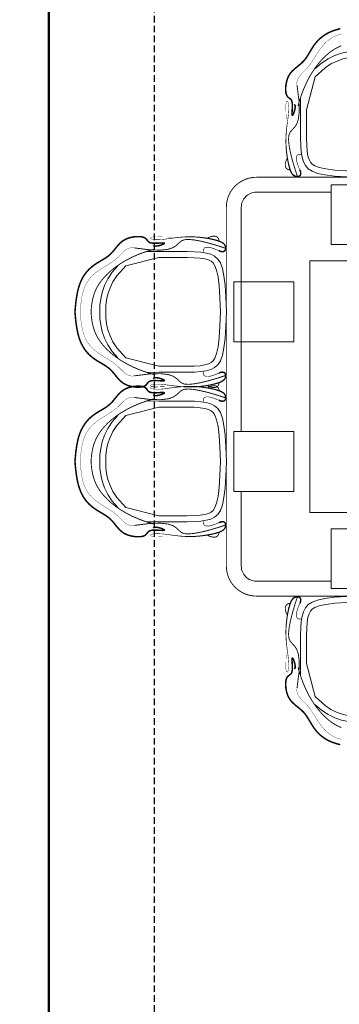
# Model space of a CAD drawing. Units: inches. Extents: x 513 to 1142, y 396 to 927.
# Tile 20 of 31: x 838 to 862, y 691 to 766. Entities that reach past the tile are written whole.
import ezdxf

# ---------------------------------------------------------------- set-up
doc = ezdxf.new("R2010")
doc.units = ezdxf.units.IN
doc.header["$MEASUREMENT"] = 0
doc.linetypes.add('DASHED', pattern=[0.75, 0.5, -0.25])
for name, color, linetype, lineweight in [('A-ANNO-DIMS', 2, 'DASHED', 18), ('A-WALL', 7, 'Continuous', 50), ('furniture', 92, 'Continuous', 18)]:
    doc.layers.add(name, color=color, linetype=linetype, lineweight=lineweight)
doc.styles.get("Standard").update_dxf_attribs({"font": 'arial.ttf'})
doc.dimstyles.get("Standard").update_dxf_attribs({"dimtxt": 4, "dimasz": 0.18, "dimexe": 0.18, "dimexo": 0.0625, "dimgap": 0.09, "dimtad": 0, "dimtih": 1, "dimtoh": 1, "dimdec": 0, "dimrnd": 6, "dimzin": 0, "dimdsep": 46, "dimlunit": 3, "dimtxsty": 'Standard', "dimcen": 0.09, "dimadec": 0, "dimazin": 0, "dimtfac": 1, "dimtdec": 0, "dimtofl": 0, "dimtmove": 0, "dimatfit": 3, "dimfxl": 1, "dimtolj": 1, "dimtzin": 0, "dimarcsym": 0})

# ---------------------------------------------------------------- blocks, each defined once
blk = doc.blocks.new('ОГ55_на6персон_стол1400х900')
for points, const_width in [([(-473.4, 523.4), (-471.2, 521.4), (-470.1, 518.2), (-469.9, 514.2), (-470.4, 509.6), (-471.4, 504.8), (-472.7, 500.1), (-474.2, 495.7), (-475.7, 492), (-477, 489.2), (-478, 487.3), (-478.9, 486.4), (-479.6, 486.4), (-480.1, 487.3), (-480.4, 489.1), (-480.6, 491.8), (-480.5, 495.4), (-480.3, 499.8), (-480, 504.9), (-479.7, 510.3), (-479.6, 516), (-479.6, 521.5), (-479.9, 526.8), (-480.6, 531.5), (-481.8, 535.5), (-483.5, 538.5), (-485.7, 540.8), (-488.2, 542.8), (-490.8, 544.6), (-493.4, 546.7), (-495.9, 549.3), (-498.1, 552.7), (-499.8, 557.2), (-501.1, 563.1), (-501.7, 570.2), (-501.7, 578.1), (-501, 586.6), (-499.6, 595.4), (-497.4, 604.2), (-494.3, 612.7), (-490.4, 620.6), (-485.5, 627.7), (-480, 634.2), (-473.9, 640.1), (-467.5, 645.6), (-460.9, 650.9), (-454.3, 656.2), (-448.1, 661.7), (-442.2, 667.5), (-436.9, 673.7), (-432.1, 680.3), (-427.6, 687.3), (-423.2, 694.5), (-418.9, 701.9), (-414.4, 709.4), (-409.5, 716.9), (-404.2, 724.4), (-398.3, 731.7), (-391.7, 738.8), (-384.3, 745.6), (-376.1, 752), (-366.9, 758), (-356.7, 763.4), (-345.4, 768.3), (-333, 772.5), (-319.5, 776), (-305.4, 778.8), (-291.5, 780.9), (-278.6, 782.6), (-267.2, 783.7), (-258.2, 784.5), (-252.2, 784.9), (-250, 785)], 5), ([(-463.8, 586.5), (-464.6, 595.2), (-463.4, 603), (-460.5, 610.1), (-456.3, 616.6), (-451.1, 622.8), (-445.3, 628.7), (-439.3, 634.6), (-433.4, 640.6), (-427.9, 646.8), (-422.8, 653.3), (-417.9, 659.9), (-413.3, 666.7), (-408.8, 673.7), (-404.4, 680.7), (-400, 687.9), (-395.5, 695), (-390.8, 702.2), (-385.8, 709.3), (-380.5, 716.3), (-374.7, 723.1), (-368.5, 729.6), (-361.7, 735.7), (-354.1, 741.4), (-345.9, 746.6), (-336.7, 751.2), (-326.7, 755.2), (-315.5, 758.7), (-303.3, 761.5), (-289.8, 763.8), (-274.9, 765.6), (-258.6, 766.8), (-250, 767.1)], 1), ([(-26.6, 523.4), (-28.8, 521.4), (-29.9, 518.2), (-30.1, 514.2), (-29.6, 509.6), (-28.6, 504.8), (-27.3, 500.1), (-25.8, 495.7), (-24.3, 492), (-23, 489.2), (-22, 487.3), (-21.1, 486.4), (-20.4, 486.4), (-19.9, 487.3), (-19.6, 489.1), (-19.4, 491.8), (-19.5, 495.4), (-19.7, 499.8), (-20, 504.9), (-20.3, 510.3), (-20.4, 516), (-20.4, 521.5), (-20.1, 526.8), (-19.4, 531.5), (-18.2, 535.5), (-16.5, 538.5), (-14.3, 540.8), (-11.8, 542.8), (-9.2, 544.6), (-6.6, 546.7), (-4.1, 549.3), (-1.9, 552.7), (-0.2, 557.2), (1.1, 563.1), (1.7, 570.2), (1.7, 578.1), (1, 586.6), (-0.4, 595.4), (-2.6, 604.2), (-5.7, 612.7), (-9.6, 620.6), (-14.5, 627.7), (-20, 634.2), (-26.1, 640.1), (-32.5, 645.6), (-39.1, 650.9), (-45.7, 656.2), (-51.9, 661.7), (-57.8, 667.5), (-63.1, 673.7), (-67.9, 680.3), (-72.4, 687.3), (-76.8, 694.5), (-81.1, 701.9), (-85.6, 709.4), (-90.5, 716.9), (-95.8, 724.4), (-101.7, 731.7), (-108.3, 738.8), (-115.7, 745.6), (-123.9, 752), (-133.1, 758), (-143.3, 763.4), (-154.6, 768.3), (-167, 772.5), (-180.5, 776), (-194.6, 778.8), (-208.5, 780.9), (-221.4, 782.6), (-232.8, 783.7), (-241.8, 784.5), (-247.8, 784.9), (-250, 785)], 5), ([(-36.2, 586.5), (-35.4, 595.2), (-36.6, 603), (-39.5, 610.1), (-43.7, 616.6), (-48.9, 622.8), (-54.7, 628.7), (-60.7, 634.6), (-66.6, 640.6), (-72.1, 646.8), (-77.2, 653.3), (-82.1, 659.9), (-86.7, 666.7), (-91.2, 673.7), (-95.6, 680.7), (-100, 687.9), (-104.5, 695), (-109.2, 702.2), (-114.2, 709.3), (-119.5, 716.3), (-125.3, 723.1), (-131.5, 729.6), (-138.3, 735.7), (-145.9, 741.4), (-154.1, 746.6), (-163.3, 751.2), (-173.3, 755.2), (-184.5, 758.7), (-196.7, 761.5), (-210.2, 763.8), (-225.1, 765.6), (-241.4, 766.8), (-250, 767.1)], 1), ([(26.6, 523.4), (28.8, 521.4), (29.9, 518.2), (30.1, 514.2), (29.6, 509.6), (28.6, 504.8), (27.3, 500.1), (25.8, 495.7), (24.3, 492), (23, 489.2), (22, 487.3), (21.1, 486.4), (20.4, 486.4), (19.9, 487.3), (19.6, 489.1), (19.4, 491.8), (19.5, 495.4), (19.7, 499.8), (20, 504.9), (20.3, 510.3), (20.4, 516), (20.4, 521.5), (20.1, 526.8), (19.4, 531.5), (18.2, 535.5), (16.5, 538.5), (14.3, 540.8), (11.8, 542.8), (9.2, 544.6), (6.6, 546.7), (4.1, 549.3), (1.9, 552.7), (0.2, 557.2), (-1.1, 563.1), (-1.7, 570.2), (-1.7, 578.1), (-1, 586.6), (0.4, 595.4), (2.6, 604.2), (5.7, 612.7), (9.6, 620.6), (14.5, 627.7), (20, 634.2), (26.1, 640.1), (32.5, 645.6), (39.1, 650.9), (45.7, 656.2), (51.9, 661.7), (57.8, 667.5), (63.1, 673.7), (67.9, 680.3), (72.4, 687.3), (76.8, 694.5), (81.1, 701.9), (85.6, 709.4), (90.5, 716.9), (95.8, 724.4), (101.7, 731.7), (108.3, 738.8), (115.7, 745.6), (123.9, 752), (133.1, 758), (143.3, 763.4), (154.6, 768.3), (167, 772.5), (180.5, 776), (194.6, 778.8), (208.5, 780.9), (221.4, 782.6), (232.8, 783.7), (241.8, 784.5), (247.8, 784.9), (250, 785)], 5), ([(36.2, 586.5), (35.4, 595.2), (36.6, 603), (39.5, 610.1), (43.7, 616.6), (48.9, 622.8), (54.7, 628.7), (60.7, 634.6), (66.6, 640.6), (72.1, 646.8), (77.2, 653.3), (82.1, 659.9), (86.7, 666.7), (91.2, 673.7), (95.6, 680.7), (100, 687.9), (104.5, 695), (109.2, 702.2), (114.2, 709.3), (119.5, 716.3), (125.3, 723.1), (131.5, 729.6), (138.3, 735.7), (145.9, 741.4), (154.1, 746.6), (163.3, 751.2), (173.3, 755.2), (184.5, 758.7), (196.7, 761.5), (210.2, 763.8), (225.1, 765.6), (241.4, 766.8), (250, 767.1)], 1), ([(473.4, 523.4), (471.2, 521.4), (470.1, 518.2), (469.9, 514.2), (470.4, 509.6), (471.4, 504.8), (472.7, 500.1), (474.2, 495.7), (475.7, 492), (477, 489.2), (478, 487.3), (478.9, 486.4), (479.6, 486.4), (480.1, 487.3), (480.4, 489.1), (480.6, 491.8), (480.5, 495.4), (480.3, 499.8), (480, 504.9), (479.7, 510.3), (479.6, 516), (479.6, 521.5), (479.9, 526.8), (480.6, 531.5), (481.8, 535.5), (483.5, 538.5), (485.7, 540.8), (488.2, 542.8), (490.8, 544.6), (493.4, 546.7), (495.9, 549.3), (498.1, 552.7), (499.8, 557.2), (501.1, 563.1), (501.7, 570.2), (501.7, 578.1), (501, 586.6), (499.6, 595.4), (497.4, 604.2), (494.3, 612.7), (490.4, 620.6), (485.5, 627.7), (480, 634.2), (473.9, 640.1), (467.5, 645.6), (460.9, 650.9), (454.3, 656.2), (448.1, 661.7), (442.2, 667.5), (436.9, 673.7), (432.1, 680.3), (427.6, 687.3), (423.2, 694.5), (418.9, 701.9), (414.4, 709.4), (409.5, 716.9), (404.2, 724.4), (398.3, 731.7), (391.7, 738.8), (384.3, 745.6), (376.1, 752), (366.9, 758), (356.7, 763.4), (345.4, 768.3), (333, 772.5), (319.5, 776), (305.4, 778.8), (291.5, 780.9), (278.6, 782.6), (267.2, 783.7), (258.2, 784.5), (252.2, 784.9), (250, 785)], 5), ([(463.8, 586.5), (464.6, 595.2), (463.4, 603), (460.5, 610.1), (456.3, 616.6), (451.1, 622.8), (445.3, 628.7), (439.3, 634.6), (433.4, 640.6), (427.9, 646.8), (422.8, 653.3), (417.9, 659.9), (413.3, 666.7), (408.8, 673.7), (404.4, 680.7), (400, 687.9), (395.5, 695), (390.8, 702.2), (385.8, 709.3), (380.5, 716.3), (374.7, 723.1), (368.5, 729.6), (361.7, 735.7), (354.1, 741.4), (345.9, 746.6), (336.7, 751.2), (326.7, 755.2), (315.5, 758.7), (303.3, 761.5), (289.8, 763.8), (274.9, 765.6), (258.6, 766.8), (250, 767.1)], 1), ([(-460.6, 517.6), (-452.3, 545.4), (-443.2, 570.7), (-433.2, 593.6), (-422.7, 614.1), (-411.8, 632.4), (-400.6, 648.7), (-389.4, 663), (-378.2, 675.4), (-367.2, 686.1), (-356.5, 695.3), (-346, 703), (-335.8, 709.4), (-325.7, 714.7), (-315.9, 718.9), (-306.4, 722.3), (-297, 724.9), (-287.9, 727), (-279.3, 728.5), (-271.3, 729.6), (-264.3, 730.4), (-258.4, 730.8), (-253.9, 731), (-251, 731.1), (-250, 731.1)], 3), ([(-39.4, 517.6), (-47.7, 545.4), (-56.8, 570.7), (-66.8, 593.6), (-77.3, 614.1), (-88.2, 632.4), (-99.4, 648.7), (-110.6, 663), (-121.8, 675.4), (-132.8, 686.1), (-143.5, 695.3), (-154, 703), (-164.2, 709.4), (-174.3, 714.7), (-184.1, 718.9), (-193.6, 722.3), (-203, 724.9), (-212.1, 727), (-220.7, 728.5), (-228.7, 729.6), (-235.7, 730.4), (-241.6, 730.8), (-246.1, 731), (-249, 731.1), (-250, 731.1)], 3), ([(39.4, 517.6), (47.7, 545.4), (56.8, 570.7), (66.8, 593.6), (77.3, 614.1), (88.2, 632.4), (99.4, 648.7), (110.6, 663), (121.8, 675.4), (132.8, 686.1), (143.5, 695.3), (154, 703), (164.2, 709.4), (174.3, 714.7), (184.1, 718.9), (193.6, 722.3), (203, 724.9), (212.1, 727), (220.7, 728.5), (228.7, 729.6), (235.7, 730.4), (241.6, 730.8), (246.1, 731), (249, 731.1), (250, 731.1)], 3), ([(460.6, 517.6), (452.3, 545.4), (443.2, 570.7), (433.2, 593.6), (422.7, 614.1), (411.8, 632.4), (400.6, 648.7), (389.4, 663), (378.2, 675.4), (367.2, 686.1), (356.5, 695.3), (346, 703), (335.8, 709.4), (325.7, 714.7), (315.9, 718.9), (306.4, 722.3), (297, 724.9), (287.9, 727), (279.3, 728.5), (271.3, 729.6), (264.3, 730.4), (258.4, 730.8), (253.9, 731), (251, 731.1), (250, 731.1)], 3), ([(-463.8, 586.5), (-457.4, 535.5), (-456.4, 498.8), (-459.4, 473.4), (-465.3, 456.6), (-472.6, 445.7), (-480.2, 437.8), (-486.8, 430.2), (-491.2, 420), (-492.3, 405.3), (-490.5, 386.7), (-486.7, 366), (-481.6, 344.5), (-475.9, 323.8), (-470.3, 305.4), (-465.6, 291), (-462.5, 281.9)], 3), ([(-36.2, 586.5), (-42.6, 535.5), (-43.6, 498.8), (-40.6, 473.4), (-34.7, 456.6), (-27.4, 445.7), (-19.8, 437.8), (-13.2, 430.2), (-8.8, 420), (-7.7, 405.3), (-9.5, 386.7), (-13.3, 366), (-18.4, 344.5), (-24.1, 323.8), (-29.7, 305.4), (-34.4, 291), (-37.5, 281.9)], 3), ([(36.2, 586.5), (42.6, 535.5), (43.6, 498.8), (40.6, 473.4), (34.7, 456.6), (27.4, 445.7), (19.8, 437.8), (13.2, 430.2), (8.8, 420), (7.7, 405.3), (9.5, 386.7), (13.3, 366), (18.4, 344.5), (24.1, 323.8), (29.7, 305.4), (34.4, 291), (37.5, 281.9)], 3), ([(463.8, 586.5), (457.4, 535.5), (456.4, 498.8), (459.4, 473.4), (465.3, 456.6), (472.6, 445.7), (480.2, 437.8), (486.8, 430.2), (491.2, 420), (492.3, 405.3), (490.5, 386.7), (486.7, 366), (481.6, 344.5), (475.9, 323.8), (470.3, 305.4), (465.6, 291), (462.5, 281.9)], 3), ([(-498, 341), (-501.3, 331.8), (-503, 324.1), (-503.1, 317.8), (-501.9, 312.9), (-499.4, 309), (-495.8, 306.2), (-491.2, 304.3), (-485.7, 303.1)], 3), ([(-454.5, 304.2), (-457.8, 312), (-461.3, 321), (-464.3, 330.3), (-466.1, 339.3), (-466, 347.1), (-463.5, 353), (-457.8, 356.1), (-448.2, 355.7)], 2), ([(-45.5, 304.2), (-42.2, 312), (-38.7, 321), (-35.7, 330.3), (-33.9, 339.3), (-34, 347.1), (-36.5, 353), (-42.2, 356.1), (-51.8, 355.7)], 2), ([(-2, 341), (1.3, 331.8), (3, 324.1), (3.1, 317.8), (1.9, 312.9), (-0.6, 309), (-4.2, 306.2), (-8.8, 304.3), (-14.3, 303.1)], 3), ([(2, 341), (-1.3, 331.8), (-3, 324.1), (-3.1, 317.8), (-1.9, 312.9), (0.6, 309), (4.2, 306.2), (8.8, 304.3), (14.3, 303.1)], 3), ([(45.5, 304.2), (42.2, 312), (38.7, 321), (35.7, 330.3), (33.9, 339.3), (34, 347.1), (36.5, 353), (42.2, 356.1), (51.8, 355.7)], 2), ([(454.5, 304.2), (457.8, 312), (461.3, 321), (464.3, 330.3), (466.1, 339.3), (466, 347.1), (463.5, 353), (457.8, 356.1), (448.2, 355.7)], 2), ([(498, 341), (501.3, 331.8), (503, 324.1), (503.1, 317.8), (501.9, 312.9), (499.4, 309), (495.8, 306.2), (491.2, 304.3), (485.7, 303.1)], 3), ([(-944.1, 52.8), (-942.1, 50.6), (-938.9, 49.4), (-934.9, 49.2), (-930.3, 49.7), (-925.5, 50.7), (-920.8, 52), (-916.4, 53.5), (-912.7, 55), (-909.9, 56.3), (-908, 57.4), (-907.1, 58.2), (-907.1, 58.9), (-908, 59.4), (-909.8, 59.7), (-912.5, 59.9), (-916.1, 59.8), (-920.5, 59.6), (-925.5, 59.3), (-931, 59), (-936.6, 58.9), (-942.2, 58.9), (-947.5, 59.2), (-952.2, 59.9), (-956.2, 61.1), (-959.2, 62.9), (-961.5, 65), (-963.4, 67.5), (-965.3, 70.1), (-967.4, 72.7), (-969.9, 75.2), (-973.4, 77.4), (-977.9, 79.2), (-983.8, 80.4), (-990.9, 81.1), (-998.8, 81.1), (-1007.3, 80.4), (-1016.1, 78.9), (-1024.9, 76.7), (-1033.4, 73.6), (-1041.3, 69.7), (-1048.4, 64.9), (-1054.8, 59.3), (-1060.7, 53.2), (-1066.3, 46.8), (-1071.6, 40.2), (-1076.9, 33.7), (-1082.4, 27.4), (-1088.1, 21.5), (-1094.4, 16.2), (-1101, 11.4), (-1108, 6.9), (-1115.2, 2.5), (-1122.6, -1.8), (-1130.1, -6.3), (-1137.6, -11.1), (-1145, -16.4), (-1152.3, -22.3), (-1159.4, -29), (-1166.2, -36.3), (-1172.7, -44.6), (-1178.7, -53.8), (-1184.1, -64), (-1189, -75.2), (-1193.2, -87.7), (-1196.7, -101.2)], 5), ([(-1007.2, 43.1), (-956.2, 36.7), (-919.4, 35.7), (-894.1, 38.7), (-877.3, 44.6), (-866.4, 51.9), (-858.5, 59.6), (-850.8, 66.2), (-840.7, 70.5), (-826, 71.6), (-807.4, 69.8), (-786.6, 66), (-765.2, 60.9), (-744.5, 55.2), (-726.1, 49.6), (-711.6, 44.9), (-702.6, 41.8)], 3), ([(-761.7, 77.3), (-752.5, 80.6), (-744.8, 82.3), (-738.5, 82.4), (-733.5, 81.2), (-729.7, 78.7), (-726.9, 75.1), (-725, 70.5), (-723.8, 65)], 3), ([(1007.2, 43.1), (956.2, 36.7), (919.4, 35.7), (894.1, 38.7), (877.3, 44.6), (866.4, 51.9), (858.5, 59.6), (850.8, 66.2), (840.7, 70.5), (826, 71.6), (807.4, 69.8), (786.6, 66), (765.2, 60.9), (744.5, 55.2), (726.1, 49.6), (711.6, 44.9), (702.6, 41.8)], 3), ([(761.7, 77.3), (752.5, 80.6), (744.8, 82.3), (738.5, 82.4), (733.5, 81.2), (729.7, 78.7), (726.9, 75.1), (725, 70.5), (723.8, 65)], 3), ([(944.1, 52.8), (942.1, 50.6), (938.9, 49.4), (934.9, 49.2), (930.3, 49.7), (925.5, 50.7), (920.8, 52), (916.4, 53.5), (912.7, 55), (909.9, 56.3), (908, 57.4), (907.1, 58.2), (907.1, 58.9), (908, 59.4), (909.8, 59.7), (912.5, 59.9), (916.1, 59.8), (920.5, 59.6), (925.5, 59.3), (931, 59), (936.6, 58.9), (942.2, 58.9), (947.5, 59.2), (952.2, 59.9), (956.2, 61.1), (959.2, 62.9), (961.5, 65), (963.4, 67.5), (965.3, 70.1), (967.4, 72.7), (969.9, 75.2), (973.4, 77.4), (977.9, 79.2), (983.8, 80.4), (990.9, 81.1), (998.8, 81.1), (1007.3, 80.4), (1016.1, 78.9), (1024.9, 76.7), (1033.4, 73.6), (1041.3, 69.7), (1048.4, 64.9), (1054.8, 59.3), (1060.7, 53.2), (1066.3, 46.8), (1071.6, 40.2), (1076.9, 33.7), (1082.4, 27.4), (1088.1, 21.5), (1094.4, 16.2), (1101, 11.4), (1108, 6.9), (1115.2, 2.5), (1122.6, -1.8), (1130.1, -6.3), (1137.6, -11.1), (1145, -16.4), (1152.3, -22.3), (1159.4, -29), (1166.2, -36.3), (1172.7, -44.6), (1178.7, -53.8), (1184.1, -64), (1189, -75.2), (1193.2, -87.7), (1196.7, -101.2)], 5), ([(-1007.2, 43.1), (-1015.9, 43.9), (-1023.6, 42.7), (-1030.7, 39.8), (-1037.3, 35.6), (-1043.5, 30.4), (-1049.4, 24.7), (-1055.3, 18.6), (-1061.3, 12.7), (-1067.5, 7.2), (-1073.9, 2.1), (-1080.6, -2.8), (-1087.4, -7.4), (-1094.3, -11.8), (-1101.4, -16.3), (-1108.5, -20.7), (-1115.7, -25.2), (-1122.9, -29.9), (-1130, -34.9), (-1137, -40.2), (-1143.8, -45.9), (-1150.3, -52.2), (-1156.4, -59), (-1162.1, -66.5), (-1167.3, -74.8), (-1171.9, -83.9), (-1175.9, -94), (-1179.3, -105.1)], 1), ([(-938.3, 40), (-966.1, 31.7), (-991.4, 22.5), (-1014.2, 12.5), (-1034.8, 2), (-1053.1, -8.9), (-1069.4, -20.1), (-1083.7, -31.3), (-1096.1, -42.5), (-1106.8, -53.5), (-1116, -64.2), (-1123.7, -74.7), (-1130.1, -84.9), (-1135.3, -94.9), (-1139.6, -104.7)], 3), ([(-724.9, 33.8), (-732.7, 37.2), (-741.6, 40.7), (-751, 43.6), (-760, 45.4), (-767.8, 45.4), (-773.6, 42.8), (-776.8, 37.1), (-776.4, 27.6)], 2), ([(724.9, 33.8), (732.7, 37.2), (741.6, 40.7), (751, 43.6), (760, 45.4), (767.8, 45.4), (773.6, 42.8), (776.8, 37.1), (776.4, 27.6)], 2), ([(938.3, 40), (966.1, 31.7), (991.4, 22.5), (1014.2, 12.5), (1034.8, 2), (1053.1, -8.9), (1069.4, -20.1), (1083.7, -31.3), (1096.1, -42.5), (1106.8, -53.5), (1116, -64.2), (1123.7, -74.7), (1130.1, -84.9), (1135.3, -94.9), (1139.6, -104.7)], 3), ([(1007.2, 43.1), (1015.9, 43.9), (1023.6, 42.7), (1030.7, 39.8), (1037.3, 35.6), (1043.5, 30.4), (1049.4, 24.7), (1055.3, 18.6), (1061.3, 12.7), (1067.5, 7.2), (1073.9, 2.1), (1080.6, -2.8), (1087.4, -7.4), (1094.3, -11.8), (1101.4, -16.3), (1108.5, -20.7), (1115.7, -25.2), (1122.9, -29.9), (1130, -34.9), (1137, -40.2), (1143.8, -45.9), (1150.3, -52.2), (1156.4, -59), (1162.1, -66.5), (1167.3, -74.8), (1171.9, -83.9), (1175.9, -94), (1179.3, -105.1)], 1)]:
    blk.add_lwpolyline(points, dxfattribs=dict(const_width=const_width))
for points in [[(-404, 641.6), (-382.6, 660.8), (-360.4, 675.6), (-337.8, 686.5), (-315.2, 694.2), (-293.1, 699), (-272, 701.6), (-252.3, 702.5), (-250, 702.4)], [(-96, 641.6), (-117.4, 660.8), (-139.6, 675.6), (-162.2, 686.5), (-184.8, 694.2), (-206.9, 699), (-228, 701.6), (-247.7, 702.5), (-250, 702.4)], [(96, 641.6), (117.4, 660.8), (139.6, 675.6), (162.2, 686.5), (184.8, 694.2), (206.9, 699), (228, 701.6), (247.7, 702.5), (250, 702.4)], [(404, 641.6), (382.6, 660.8), (360.4, 675.6), (337.8, 686.5), (315.2, 694.2), (293.1, 699), (272, 701.6), (252.3, 702.5), (250, 702.4)], [(-403.6, 615), (-370.3, 644.9), (-350.5, 658.2), (-330.2, 668), (-309.8, 674.9), (-289.8, 679.3), (-270.4, 681.7), (-252.1, 682.5), (-250.4, 682.4)], [(-96.4, 615), (-129.7, 644.9), (-149.5, 658.2), (-169.8, 668), (-190.2, 674.9), (-210.2, 679.3), (-229.6, 681.7), (-247.9, 682.5), (-249.6, 682.4)], [(96.4, 615), (129.7, 644.9), (149.5, 658.2), (169.8, 668), (190.2, 674.9), (210.2, 679.3), (229.6, 681.7), (247.9, 682.5), (249.6, 682.4)], [(403.6, 615), (370.3, 644.9), (350.5, 658.2), (330.2, 668), (309.8, 674.9), (289.8, 679.3), (270.4, 681.7), (252.1, 682.5), (250.4, 682.4)], [(-403.6, 615), (-431.9, 505.2), (-431.9, 469.2), (-432, 437.6), (-431.9, 410.1), (-431.2, 386.6), (-429.8, 367), (-427.3, 351.1), (-423.8, 338.8), (-419.4, 329.9), (-413.6, 323.3), (-404.4, 317.4), (-389.5, 311.8), (-367.3, 307), (-337.1, 303.4), (-298.1, 300.9), (-249.4, 299.3)], [(-96.4, 615), (-68.1, 505.2), (-68.1, 469.2), (-68, 437.6), (-68.1, 410.1), (-68.8, 386.6), (-70.2, 367), (-72.7, 351.1), (-76.2, 338.8), (-80.6, 329.9), (-86.4, 323.3), (-95.6, 317.4), (-110.5, 311.8), (-132.7, 307), (-162.9, 303.4), (-201.9, 300.9), (-250.6, 299.3)], [(96.4, 615), (68.1, 505.2), (68.1, 469.2), (68, 437.6), (68.1, 410.1), (68.8, 386.6), (70.2, 367), (72.7, 351.1), (76.2, 338.8), (80.6, 329.9), (86.4, 323.3), (95.6, 317.4), (110.5, 311.8), (132.7, 307), (162.9, 303.4), (201.9, 300.9), (250.6, 299.3)], [(403.6, 615), (431.9, 505.2), (431.9, 469.2), (432, 437.6), (431.9, 410.1), (431.2, 386.6), (429.8, 367), (427.3, 351.1), (423.8, 338.8), (419.4, 329.9), (413.6, 323.3), (404.4, 317.4), (389.5, 311.8), (367.3, 307), (337.1, 303.4), (298.1, 300.9), (249.4, 299.3)], [(-452.3, 545.4), (-451.9, 505.1), (-451.9, 469.2), (-452, 437.5), (-451.9, 409.8), (-451.2, 385.6), (-449.6, 364.7), (-446.8, 346.8), (-442.5, 331.5), (-436.1, 318.7), (-426.8, 308), (-413.5, 299.4), (-395.1, 292.5), (-370.6, 287.3), (-339, 283.5), (-299.1, 280.9), (-250, 279.3)], [(-47.7, 545.4), (-48.1, 505.1), (-48.1, 469.2), (-48, 437.5), (-48.1, 409.8), (-48.8, 385.6), (-50.4, 364.7), (-53.2, 346.8), (-57.5, 331.5), (-63.9, 318.7), (-73.2, 308), (-86.5, 299.4), (-104.9, 292.5), (-129.4, 287.3), (-161, 283.5), (-200.9, 280.9), (-250, 279.3)], [(47.7, 545.4), (48.1, 505.1), (48.1, 469.2), (48, 437.5), (48.1, 409.8), (48.8, 385.6), (50.4, 364.7), (53.2, 346.8), (57.5, 331.5), (63.9, 318.7), (73.2, 308), (86.5, 299.4), (104.9, 292.5), (129.4, 287.3), (161, 283.5), (200.9, 280.9), (250, 279.3)], [(452.3, 545.4), (451.9, 505.1), (451.9, 469.2), (452, 437.5), (451.9, 409.8), (451.2, 385.6), (449.6, 364.7), (446.8, 346.8), (442.5, 331.5), (436.1, 318.7), (426.8, 308), (413.5, 299.4), (395.1, 292.5), (370.6, 287.3), (339, 283.5), (299.1, 280.9), (250, 279.3)], [(-1035.7, -17.1), (-925.9, 11.2), (-889.9, 11.2), (-858.2, 11.3), (-830.8, 11.2), (-807.3, 10.5), (-787.6, 9.1), (-771.7, 6.6), (-759.5, 3.1), (-750.6, -1.3), (-744, -7.1), (-738, -16.3), (-732.5, -31.2), (-727.7, -53.4), (-724.1, -83.6), (-721.5, -122.5), (-720, -171.3)], [(-966.1, 31.7), (-925.8, 31.2), (-889.9, 31.2), (-858.2, 31.3), (-830.4, 31.2), (-806.3, 30.5), (-785.4, 29), (-767.4, 26.2), (-752.2, 21.8), (-739.4, 15.4), (-728.7, 6.1), (-720.1, -7.2), (-713.2, -25.6), (-708, -50.1), (-704.2, -81.7), (-701.6, -121.6), (-700, -170.7)], [(966.1, 31.7), (925.8, 31.2), (889.9, 31.2), (858.2, 31.3), (830.4, 31.2), (806.3, 30.5), (785.4, 29), (767.4, 26.2), (752.2, 21.8), (739.4, 15.4), (728.7, 6.1), (720.1, -7.2), (713.2, -25.6), (708, -50.1), (704.2, -81.7), (701.6, -121.6), (700, -170.7)], [(1035.7, -17.1), (925.9, 11.2), (889.9, 11.2), (858.2, 11.3), (830.8, 11.2), (807.3, 10.5), (787.6, 9.1), (771.7, 6.6), (759.5, 3.1), (750.6, -1.3), (744, -7.1), (738, -16.3), (732.5, -31.2), (727.7, -53.4), (724.1, -83.6), (721.5, -122.5), (720, -171.3)], [(-1062.3, -16.7), (-1081.4, -38.1), (-1096.2, -60.3), (-1107.2, -82.9), (-1114.8, -105.5), (-1119.7, -127.5), (-1122.3, -148.6), (-1123.1, -168.3), (-1123.1, -170.7)], [(-1035.7, -17.1), (-1065.6, -50.4), (-1078.8, -70.2), (-1088.7, -90.5), (-1095.5, -110.8), (-1100, -130.9), (-1102.3, -150.3), (-1103.1, -168.6), (-1103.1, -170.3)], [(1035.7, -17.1), (1065.6, -50.4), (1078.8, -70.2), (1088.7, -90.5), (1095.5, -110.8), (1100, -130.9), (1102.3, -150.3), (1103.1, -168.6), (1103.1, -170.3)], [(1062.3, -16.7), (1081.4, -38.1), (1096.2, -60.3), (1107.2, -82.9), (1114.8, -105.5), (1119.7, -127.5), (1122.3, -148.6), (1123.1, -168.3), (1123.1, -170.7)]]:
    blk.add_lwpolyline(points)
for points, format in [([(-454.5, 304.2, 5, 4.91, 0), (-452, 297.4, 4.91, 4.84, 0), (-451.3, 292.1, 4.84, 4.78, 0), (-451.9, 288.1, 4.78, 4.74, 0), (-453.7, 285.1, 4.74, 4.7, 0), (-456.3, 283.2, 4.7, 4.65, 0), (-459.4, 282.2, 4.65, 4.61, 0), (-462.9, 281.8, 4.61, 4.56, 0), (-466.5, 282.1, 4.56, 4.52, 0), (-469.8, 282.8, 4.52, 4.47, 0), (-472.9, 284.1, 4.47, 4.43, 0), (-475.9, 286.1, 4.43, 4.38, 0), (-478.7, 288.8, 4.38, 4.32, 0), (-481.3, 292.5, 4.32, 4.25, 0), (-483.8, 297.3, 4.25, 4.17, 0), (-486.3, 303.2, 4.17, 4.07, 0), (-488.7, 310.4, 4.07, 3.95, 0), (-491, 318.9, 3.95, 3.82, 0), (-493.3, 328.7, 3.82, 3.68, 0), (-495.4, 339.4, 3.68, 3.53, 0), (-497.2, 350.9, 3.53, 3.37, 0), (-498.8, 363, 3.37, 3.21, 0), (-500, 375.5, 3.21, 3.05, 0), (-500.8, 388.2, 3.05, 2.88, 0), (-501.1, 400.7, 2.88, 2.72, 0), (-500.9, 413.1, 2.72, 2.57, 0), (-500.2, 425.1, 2.57, 2.41, 0), (-499.2, 436.7, 2.41, 2.27, 0), (-498, 447.8, 2.27, 2.13, 0), (-496.7, 458.3, 2.13, 2, 0), (-495.3, 468.2, 2, 1.88, 0), (-494.1, 477.3, 1.88, 1.78, 0), (-493, 485.6, 1.78, 1.68, 0), (-492.2, 493.1, 1.68, 1.59, 0), (-491.7, 499.6, 1.59, 1.52, 0), (-491.4, 505.4, 1.52, 1.45, 0), (-491.3, 510.5, 1.45, 1.4, 0), (-491.4, 514.9, 1.4, 1.35, 0), (-491.6, 518.7, 1.35, 1.3, 0), (-492, 521.9, 1.3, 1.27, 0), (-492.4, 524.7, 1.27, 1.24, 0), (-492.8, 527, 1.24, 1.21, 0), (-493.3, 528.8, 1.21, 1.19, 0), (-493.8, 530.3, 1.19, 1.18, 0), (-494.3, 531.5, 1.18, 1.16, 0), (-494.8, 532.3, 1.16, 1.15, 0), (-495.3, 532.9, 1.15, 1.14, 0), (-495.8, 533.2, 1.14, 1.14, 0), (-496.3, 533.3, 1.14, 1.13, 0), (-496.8, 533.2, 1.13, 1.12, 0), (-497.3, 533, 1.12, 1.12, 0), (-497.8, 532.5, 1.12, 1.11, 0), (-498.3, 531.9, 1.11, 1.09, 0), (-498.7, 531.1, 1.09, 1.08, 0), (-499.1, 530.2, 1.08, 1.07, 0), (-499.5, 529.1, 1.07, 1.05, 0), (-499.9, 527.9, 1.05, 1.03, 0), (-500.3, 526.5, 1.03, 1.01, 0), (-500.6, 524.9, 1.01, 0.986, 0), (-500.9, 523.1, 0.986, 0.959, 0), (-501.1, 521, 0.959, 0.926, 0), (-501.3, 518.5, 0.926, 0.889, 0), (-501.4, 515.7, 0.889, 0.846, 0), (-501.4, 512.3, 0.846, 0.796, 0), (-501.3, 508.5, 0.796, 0.738, 0), (-501.1, 504, 0.738, 0.672, 0), (-500.8, 498.9, 0.672, 0.595, 0), (-500.6, 493, 0.595, 0.506, 0), (-500.3, 486.1, 0.506, 0.404, 0), (-500.1, 478.2, 0.404, 0.286, 0), (-499.9, 469.2, 0.286, 0.152, 0), (-499.9, 458.8, 0.152, 0, 0), (-500, 447.1, 0, 0, 0)], "xyseb"), ([(-45.5, 304.2, 5, 4.91, 0), (-48, 297.4, 4.91, 4.84, 0), (-48.7, 292.1, 4.84, 4.78, 0), (-48.1, 288.1, 4.78, 4.74, 0), (-46.3, 285.1, 4.74, 4.7, 0), (-43.7, 283.2, 4.7, 4.65, 0), (-40.6, 282.2, 4.65, 4.61, 0), (-37.1, 281.8, 4.61, 4.56, 0), (-33.5, 282.1, 4.56, 4.52, 0), (-30.2, 282.8, 4.52, 4.47, 0), (-27.1, 284.1, 4.47, 4.43, 0), (-24.1, 286.1, 4.43, 4.38, 0), (-21.3, 288.8, 4.38, 4.32, 0), (-18.7, 292.5, 4.32, 4.25, 0), (-16.2, 297.3, 4.25, 4.17, 0), (-13.7, 303.2, 4.17, 4.07, 0), (-11.3, 310.4, 4.07, 3.95, 0), (-9, 318.9, 3.95, 3.82, 0), (-6.7, 328.7, 3.82, 3.68, 0), (-4.6, 339.4, 3.68, 3.53, 0), (-2.8, 350.9, 3.53, 3.37, 0), (-1.2, 363, 3.37, 3.21, 0), (0, 375.5, 3.21, 3.05, 0), (0.8, 388.2, 3.05, 2.88, 0), (1.1, 400.7, 2.88, 2.72, 0), (0.9, 413.1, 2.72, 2.57, 0), (0.2, 425.1, 2.57, 2.41, 0), (-0.8, 436.7, 2.41, 2.27, 0), (-2, 447.8, 2.27, 2.13, 0), (-3.3, 458.3, 2.13, 2, 0), (-4.7, 468.2, 2, 1.88, 0), (-5.9, 477.3, 1.88, 1.78, 0), (-7, 485.6, 1.78, 1.68, 0), (-7.8, 493.1, 1.68, 1.59, 0), (-8.3, 499.6, 1.59, 1.52, 0), (-8.6, 505.4, 1.52, 1.45, 0), (-8.7, 510.5, 1.45, 1.4, 0), (-8.6, 514.9, 1.4, 1.35, 0), (-8.4, 518.7, 1.35, 1.3, 0), (-8, 521.9, 1.3, 1.27, 0), (-7.6, 524.7, 1.27, 1.24, 0), (-7.2, 527, 1.24, 1.21, 0), (-6.7, 528.8, 1.21, 1.19, 0), (-6.2, 530.3, 1.19, 1.18, 0), (-5.7, 531.5, 1.18, 1.16, 0), (-5.2, 532.3, 1.16, 1.15, 0), (-4.7, 532.9, 1.15, 1.14, 0), (-4.2, 533.2, 1.14, 1.14, 0), (-3.7, 533.3, 1.14, 1.13, 0), (-3.2, 533.2, 1.13, 1.12, 0), (-2.7, 533, 1.12, 1.12, 0), (-2.2, 532.5, 1.12, 1.11, 0), (-1.7, 531.9, 1.11, 1.09, 0), (-1.3, 531.1, 1.09, 1.08, 0), (-0.9, 530.2, 1.08, 1.07, 0), (-0.5, 529.1, 1.07, 1.05, 0), (-0.1, 527.9, 1.05, 1.03, 0), (0.3, 526.5, 1.03, 1.01, 0), (0.6, 524.9, 1.01, 0.986, 0), (0.9, 523.1, 0.986, 0.959, 0), (1.1, 521, 0.959, 0.926, 0), (1.3, 518.5, 0.926, 0.889, 0), (1.4, 515.7, 0.889, 0.846, 0), (1.4, 512.3, 0.846, 0.796, 0), (1.3, 508.5, 0.796, 0.738, 0), (1.1, 504, 0.738, 0.672, 0), (0.8, 498.9, 0.672, 0.595, 0), (0.6, 493, 0.595, 0.506, 0), (0.3, 486.1, 0.506, 0.404, 0), (0.1, 478.2, 0.404, 0.286, 0), (-0.1, 469.2, 0.286, 0.152, 0), (-0.1, 458.8, 0.152, 0, 0), (0, 447.1, 0, 0, 0)], "xyseb"), ([(45.5, 304.2, 5, 4.91, 0), (48, 297.4, 4.91, 4.84, 0), (48.7, 292.1, 4.84, 4.78, 0), (48.1, 288.1, 4.78, 4.74, 0), (46.3, 285.1, 4.74, 4.7, 0), (43.7, 283.2, 4.7, 4.65, 0), (40.6, 282.2, 4.65, 4.61, 0), (37.1, 281.8, 4.61, 4.56, 0), (33.5, 282.1, 4.56, 4.52, 0), (30.2, 282.8, 4.52, 4.47, 0), (27.1, 284.1, 4.47, 4.43, 0), (24.1, 286.1, 4.43, 4.38, 0), (21.3, 288.8, 4.38, 4.32, 0), (18.7, 292.5, 4.32, 4.25, 0), (16.2, 297.3, 4.25, 4.17, 0), (13.7, 303.2, 4.17, 4.07, 0), (11.3, 310.4, 4.07, 3.95, 0), (9, 318.9, 3.95, 3.82, 0), (6.7, 328.7, 3.82, 3.68, 0), (4.6, 339.4, 3.68, 3.53, 0), (2.8, 350.9, 3.53, 3.37, 0), (1.2, 363, 3.37, 3.21, 0), (0, 375.5, 3.21, 3.05, 0), (-0.8, 388.2, 3.05, 2.88, 0), (-1.1, 400.7, 2.88, 2.72, 0), (-0.9, 413.1, 2.72, 2.57, 0), (-0.2, 425.1, 2.57, 2.41, 0), (0.8, 436.7, 2.41, 2.27, 0), (2, 447.8, 2.27, 2.13, 0), (3.3, 458.3, 2.13, 2, 0), (4.7, 468.2, 2, 1.88, 0), (5.9, 477.3, 1.88, 1.78, 0), (7, 485.6, 1.78, 1.68, 0), (7.8, 493.1, 1.68, 1.59, 0), (8.3, 499.6, 1.59, 1.52, 0), (8.6, 505.4, 1.52, 1.45, 0), (8.7, 510.5, 1.45, 1.4, 0), (8.6, 514.9, 1.4, 1.35, 0), (8.4, 518.7, 1.35, 1.3, 0), (8, 521.9, 1.3, 1.27, 0), (7.6, 524.7, 1.27, 1.24, 0), (7.2, 527, 1.24, 1.21, 0), (6.7, 528.8, 1.21, 1.19, 0), (6.2, 530.3, 1.19, 1.18, 0), (5.7, 531.5, 1.18, 1.16, 0), (5.2, 532.3, 1.16, 1.15, 0), (4.7, 532.9, 1.15, 1.14, 0), (4.2, 533.2, 1.14, 1.14, 0), (3.7, 533.3, 1.14, 1.13, 0), (3.2, 533.2, 1.13, 1.12, 0), (2.7, 533, 1.12, 1.12, 0), (2.2, 532.5, 1.12, 1.11, 0), (1.7, 531.9, 1.11, 1.09, 0), (1.3, 531.1, 1.09, 1.08, 0), (0.9, 530.2, 1.08, 1.07, 0), (0.5, 529.1, 1.07, 1.05, 0), (0.1, 527.9, 1.05, 1.03, 0), (-0.3, 526.5, 1.03, 1.01, 0), (-0.6, 524.9, 1.01, 0.986, 0), (-0.9, 523.1, 0.986, 0.959, 0), (-1.1, 521, 0.959, 0.926, 0), (-1.3, 518.5, 0.926, 0.889, 0), (-1.4, 515.7, 0.889, 0.846, 0), (-1.4, 512.3, 0.846, 0.796, 0), (-1.3, 508.5, 0.796, 0.738, 0), (-1.1, 504, 0.738, 0.672, 0), (-0.8, 498.9, 0.672, 0.595, 0), (-0.6, 493, 0.595, 0.506, 0), (-0.3, 486.1, 0.506, 0.404, 0), (-0.1, 478.2, 0.404, 0.286, 0), (0.1, 469.2, 0.286, 0.152, 0), (0.1, 458.8, 0.152, 0, 0), (0, 447.1, 0, 0, 0)], "xyseb"), ([(454.5, 304.2, 5, 4.91, 0), (452, 297.4, 4.91, 4.84, 0), (451.3, 292.1, 4.84, 4.78, 0), (451.9, 288.1, 4.78, 4.74, 0), (453.7, 285.1, 4.74, 4.7, 0), (456.3, 283.2, 4.7, 4.65, 0), (459.4, 282.2, 4.65, 4.61, 0), (462.9, 281.8, 4.61, 4.56, 0), (466.5, 282.1, 4.56, 4.52, 0), (469.8, 282.8, 4.52, 4.47, 0), (472.9, 284.1, 4.47, 4.43, 0), (475.9, 286.1, 4.43, 4.38, 0), (478.7, 288.8, 4.38, 4.32, 0), (481.3, 292.5, 4.32, 4.25, 0), (483.8, 297.3, 4.25, 4.17, 0), (486.3, 303.2, 4.17, 4.07, 0), (488.7, 310.4, 4.07, 3.95, 0), (491, 318.9, 3.95, 3.82, 0), (493.3, 328.7, 3.82, 3.68, 0), (495.4, 339.4, 3.68, 3.53, 0), (497.2, 350.9, 3.53, 3.37, 0), (498.8, 363, 3.37, 3.21, 0), (500, 375.5, 3.21, 3.05, 0), (500.8, 388.2, 3.05, 2.88, 0), (501.1, 400.7, 2.88, 2.72, 0), (500.9, 413.1, 2.72, 2.57, 0), (500.2, 425.1, 2.57, 2.41, 0), (499.2, 436.7, 2.41, 2.27, 0), (498, 447.8, 2.27, 2.13, 0), (496.7, 458.3, 2.13, 2, 0), (495.3, 468.2, 2, 1.88, 0), (494.1, 477.3, 1.88, 1.78, 0), (493, 485.6, 1.78, 1.68, 0), (492.2, 493.1, 1.68, 1.59, 0), (491.7, 499.6, 1.59, 1.52, 0), (491.4, 505.4, 1.52, 1.45, 0), (491.3, 510.5, 1.45, 1.4, 0), (491.4, 514.9, 1.4, 1.35, 0), (491.6, 518.7, 1.35, 1.3, 0), (492, 521.9, 1.3, 1.27, 0), (492.4, 524.7, 1.27, 1.24, 0), (492.8, 527, 1.24, 1.21, 0), (493.3, 528.8, 1.21, 1.19, 0), (493.8, 530.3, 1.19, 1.18, 0), (494.3, 531.5, 1.18, 1.16, 0), (494.8, 532.3, 1.16, 1.15, 0), (495.3, 532.9, 1.15, 1.14, 0), (495.8, 533.2, 1.14, 1.14, 0), (496.3, 533.3, 1.14, 1.13, 0), (496.8, 533.2, 1.13, 1.12, 0), (497.3, 533, 1.12, 1.12, 0), (497.8, 532.5, 1.12, 1.11, 0), (498.3, 531.9, 1.11, 1.09, 0), (498.7, 531.1, 1.09, 1.08, 0), (499.1, 530.2, 1.08, 1.07, 0), (499.5, 529.1, 1.07, 1.05, 0), (499.9, 527.9, 1.05, 1.03, 0), (500.3, 526.5, 1.03, 1.01, 0), (500.6, 524.9, 1.01, 0.986, 0), (500.9, 523.1, 0.986, 0.959, 0), (501.1, 521, 0.959, 0.926, 0), (501.3, 518.5, 0.926, 0.889, 0), (501.4, 515.7, 0.889, 0.846, 0), (501.4, 512.3, 0.846, 0.796, 0), (501.3, 508.5, 0.796, 0.738, 0), (501.1, 504, 0.738, 0.672, 0), (500.8, 498.9, 0.672, 0.595, 0), (500.6, 493, 0.595, 0.506, 0), (500.3, 486.1, 0.506, 0.404, 0), (500.1, 478.2, 0.404, 0.286, 0), (499.9, 469.2, 0.286, 0.152, 0), (499.9, 458.8, 0.152, 0, 0), (500, 447.1, 0, 0, 0)], "xyseb"), ([(-650, -70.7), (-650, 179.3, -0.414214), (-600, 229.3), (-350, 229.3)], "xyb"), ([(-150, 229.3), (600, 229.3, -0.414214), (650, 179.3), (650, -70.7)], "xyb"), ([(-724.9, 33.8, 5, 4.91, 0), (-718.1, 31.4, 4.91, 4.84, 0), (-712.8, 30.6, 4.84, 4.78, 0), (-708.7, 31.2, 4.78, 4.74, 0), (-705.8, 33, 4.74, 4.7, 0), (-703.9, 35.6, 4.7, 4.65, 0), (-702.9, 38.8, 4.65, 4.61, 0), (-702.5, 42.3, 4.61, 4.56, 0), (-702.8, 45.8, 4.56, 4.52, 0), (-703.5, 49.1, 4.52, 4.47, 0), (-704.8, 52.2, 4.47, 4.43, 0), (-706.7, 55.2, 4.43, 4.38, 0), (-709.5, 58, 4.38, 4.32, 0), (-713.2, 60.6, 4.32, 4.25, 0), (-717.9, 63.2, 4.25, 4.17, 0), (-723.8, 65.6, 4.17, 4.07, 0), (-731, 68, 4.07, 3.95, 0), (-739.6, 70.4, 3.95, 3.82, 0), (-749.3, 72.6, 3.82, 3.68, 0), (-760.1, 74.7, 3.68, 3.53, 0), (-771.6, 76.5, 3.53, 3.37, 0), (-783.7, 78.1, 3.37, 3.21, 0), (-796.2, 79.3, 3.21, 3.05, 0), (-808.8, 80.1, 3.05, 2.88, 0), (-821.4, 80.4, 2.88, 2.72, 0), (-833.8, 80.2, 2.72, 2.57, 0), (-845.8, 79.5, 2.57, 2.41, 0), (-857.4, 78.6, 2.41, 2.27, 0), (-868.5, 77.3, 2.27, 2.13, 0), (-879, 76, 2.13, 2, 0), (-888.9, 74.6, 2, 1.88, 0), (-898, 73.4, 1.88, 1.78, 0), (-906.3, 72.3, 1.78, 1.68, 0), (-913.7, 71.5, 1.68, 1.59, 0), (-920.3, 71, 1.59, 1.52, 0), (-926.1, 70.7, 1.52, 1.45, 0), (-931.2, 70.7, 1.45, 1.4, 0), (-935.6, 70.7, 1.4, 1.35, 0), (-939.4, 71, 1.35, 1.3, 0), (-942.6, 71.3, 1.3, 1.27, 0), (-945.3, 71.7, 1.27, 1.24, 0), (-947.6, 72.1, 1.24, 1.21, 0), (-949.5, 72.6, 1.21, 1.19, 0), (-951, 73.1, 1.19, 1.18, 0), (-952.2, 73.6, 1.18, 1.16, 0), (-953, 74.1, 1.16, 1.15, 0), (-953.6, 74.6, 1.15, 1.14, 0), (-953.9, 75.1, 1.14, 1.14, 0), (-954, 75.6, 1.14, 1.13, 0), (-953.9, 76.2, 1.13, 1.12, 0), (-953.6, 76.6, 1.12, 1.12, 0), (-953.2, 77.1, 1.12, 1.11, 0), (-952.6, 77.6, 1.11, 1.09, 0), (-951.8, 78, 1.09, 1.08, 0), (-950.9, 78.4, 1.08, 1.07, 0), (-949.8, 78.9, 1.07, 1.05, 0), (-948.6, 79.2, 1.05, 1.03, 0), (-947.2, 79.6, 1.03, 1.01, 0), (-945.6, 79.9, 1.01, 0.986, 0), (-943.8, 80.2, 0.986, 0.959, 0), (-941.7, 80.4, 0.959, 0.926, 0), (-939.2, 80.6, 0.926, 0.889, 0), (-936.3, 80.7, 0.889, 0.846, 0), (-933, 80.7, 0.846, 0.796, 0), (-929.1, 80.6, 0.796, 0.738, 0), (-924.7, 80.4, 0.738, 0.672, 0), (-919.6, 80.2, 0.672, 0.595, 0), (-913.7, 79.9, 0.595, 0.506, 0), (-906.8, 79.6, 0.506, 0.404, 0), (-898.9, 79.4, 0.404, 0.286, 0), (-889.9, 79.2, 0.286, 0.152, 0), (-879.5, 79.2, 0.152, 0, 0), (-867.8, 79.4, 0, 0, 0)], "xyseb"), ([(724.9, 33.8, 5, 4.91, 0), (718.1, 31.4, 4.91, 4.84, 0), (712.8, 30.6, 4.84, 4.78, 0), (708.7, 31.2, 4.78, 4.74, 0), (705.8, 33, 4.74, 4.7, 0), (703.9, 35.6, 4.7, 4.65, 0), (702.9, 38.8, 4.65, 4.61, 0), (702.5, 42.3, 4.61, 4.56, 0), (702.8, 45.8, 4.56, 4.52, 0), (703.5, 49.1, 4.52, 4.47, 0), (704.8, 52.2, 4.47, 4.43, 0), (706.7, 55.2, 4.43, 4.38, 0), (709.5, 58, 4.38, 4.32, 0), (713.2, 60.6, 4.32, 4.25, 0), (717.9, 63.2, 4.25, 4.17, 0), (723.8, 65.6, 4.17, 4.07, 0), (731, 68, 4.07, 3.95, 0), (739.6, 70.4, 3.95, 3.82, 0), (749.3, 72.6, 3.82, 3.68, 0), (760.1, 74.7, 3.68, 3.53, 0), (771.6, 76.5, 3.53, 3.37, 0), (783.7, 78.1, 3.37, 3.21, 0), (796.2, 79.3, 3.21, 3.05, 0), (808.8, 80.1, 3.05, 2.88, 0), (821.4, 80.4, 2.88, 2.72, 0), (833.8, 80.2, 2.72, 2.57, 0), (845.8, 79.5, 2.57, 2.41, 0), (857.4, 78.6, 2.41, 2.27, 0), (868.5, 77.3, 2.27, 2.13, 0), (879, 76, 2.13, 2, 0), (888.9, 74.6, 2, 1.88, 0), (898, 73.4, 1.88, 1.78, 0), (906.3, 72.3, 1.78, 1.68, 0), (913.7, 71.5, 1.68, 1.59, 0), (920.3, 71, 1.59, 1.52, 0), (926.1, 70.7, 1.52, 1.45, 0), (931.2, 70.7, 1.45, 1.4, 0), (935.6, 70.7, 1.4, 1.35, 0), (939.4, 71, 1.35, 1.3, 0), (942.6, 71.3, 1.3, 1.27, 0), (945.3, 71.7, 1.27, 1.24, 0), (947.6, 72.1, 1.24, 1.21, 0), (949.5, 72.6, 1.21, 1.19, 0), (951, 73.1, 1.19, 1.18, 0), (952.2, 73.6, 1.18, 1.16, 0), (953, 74.1, 1.16, 1.15, 0), (953.6, 74.6, 1.15, 1.14, 0), (953.9, 75.1, 1.14, 1.14, 0), (954, 75.6, 1.14, 1.13, 0), (953.9, 76.2, 1.13, 1.12, 0), (953.6, 76.6, 1.12, 1.12, 0), (953.2, 77.1, 1.12, 1.11, 0), (952.6, 77.6, 1.11, 1.09, 0), (951.8, 78, 1.09, 1.08, 0), (950.9, 78.4, 1.08, 1.07, 0), (949.8, 78.9, 1.07, 1.05, 0), (948.6, 79.2, 1.05, 1.03, 0), (947.2, 79.6, 1.03, 1.01, 0), (945.6, 79.9, 1.01, 0.986, 0), (943.8, 80.2, 0.986, 0.959, 0), (941.7, 80.4, 0.959, 0.926, 0), (939.2, 80.6, 0.926, 0.889, 0), (936.3, 80.7, 0.889, 0.846, 0), (933, 80.7, 0.846, 0.796, 0), (929.1, 80.6, 0.796, 0.738, 0), (924.7, 80.4, 0.738, 0.672, 0), (919.6, 80.2, 0.672, 0.595, 0), (913.7, 79.9, 0.595, 0.506, 0), (906.8, 79.6, 0.506, 0.404, 0), (898.9, 79.4, 0.404, 0.286, 0), (889.9, 79.2, 0.286, 0.152, 0), (879.5, 79.2, 0.152, 0, 0), (867.8, 79.4, 0, 0, 0)], "xyseb")]:
    blk.add_lwpolyline(points, format=format)
at = {"const_width": 3}
blk.add_lwpolyline([(-600, 279.3), (600, 279.3, -0.414214), (700, 179.3), (700, -520.7, -0.414214), (600, -620.7), (-600, -620.7, -0.414214), (-700, -520.7), (-700, 179.3, -0.414214)], format="xyb", close=True, dxfattribs=at)
for points in [[(-150, 254.3), (-150, 54.3), (-350, 54.3), (-350, 254.3)], [(150, 254.3), (150, 54.3), (350, 54.3), (350, 254.3)], [(-420.7, -341.4), (420.7, -341.4), (420.7, 0), (-420.7, 0)], [(-675, -270.7), (-475, -270.7), (-475, -70.7), (-675, -70.7)], [(675, -270.7), (475, -270.7), (475, -70.7), (675, -70.7)]]:
    blk.add_lwpolyline(points, close=True)
blk = doc.blocks.new('*D137')
at = {"layer": 'A-ANNO-DIMS', "color": 0, "lineweight": -2, "transparency": 16777216}
for p, q in [((839.995, 770.096), (839.995, 401.578)), ((920.995, 770.067), (920.995, 401.578)), ((840.175, 401.758), (875.078, 401.758)), ((920.815, 401.758), (885.913, 401.758))]:
    blk.add_line(p, q, dxfattribs=at)
at = {"layer": 'A-ANNO-DIMS', "color": 0, "transparency": 16777216}
for points in [[(840.175, 401.788), (840.175, 401.728), (839.995, 401.758)], [(920.815, 401.788), (920.815, 401.728), (920.995, 401.758)]]:
    blk.add_solid(points, dxfattribs=at)
at = {"layer": 'Defpoints', "color": 0, "transparency": 16777216}
for p in [(839.995, 770.158), (920.995, 770.13), (920.995, 401.758)]:
    blk.add_point(p, dxfattribs=at)
at = {"layer": 'A-ANNO-DIMS', "color": 0, "transparency": 16777216, "insert": (880.495, 401.758), "char_height": 4, "attachment_point": 5}
blk.add_mtext('\\A1;6\'-9"', dxfattribs=at)
blk = doc.blocks.new('*D149')
at = {"layer": 'A-ANNO-DIMS', "color": 0, "lineweight": -2, "transparency": 16777216}
for p, q in [((840.058, 770.158), (1131.575, 770.158)), ((1131.395, 769.978), (1131.395, 707.791)), ((1131.395, 641.338), (1131.395, 703.526)), ((840.058, 641.158), (1131.575, 641.158))]:
    blk.add_line(p, q, dxfattribs=at)
at = {"layer": 'A-ANNO-DIMS', "color": 0, "transparency": 16777216}
for points in [[(1131.365, 769.978), (1131.425, 769.978), (1131.395, 770.158)], [(1131.365, 641.338), (1131.425, 641.338), (1131.395, 641.158)]]:
    blk.add_solid(points, dxfattribs=at)
at = {"layer": 'Defpoints', "color": 0, "transparency": 16777216}
for p in [(839.995, 770.158), (1131.395, 770.158), (839.995, 641.158)]:
    blk.add_point(p, dxfattribs=at)
at = {"layer": 'A-ANNO-DIMS', "color": 0, "transparency": 16777216, "insert": (1131.395, 705.658), "char_height": 4, "attachment_point": 5}
blk.add_mtext('\\A1;10\'-9"', dxfattribs=at)
blk = doc.blocks.new('*D169')
at = {"layer": 'A-ANNO-DIMS', "color": 0, "lineweight": -2, "transparency": 16777216}
for p, q in [((835.995, 774.096), (835.995, 401.578)), ((839.995, 774.096), (839.995, 401.578)), ((836.175, 401.758), (839.815, 401.758)), ((839.995, 401.758), (840.175, 401.758))]:
    blk.add_line(p, q, dxfattribs=at)
at = {"layer": 'A-ANNO-DIMS', "color": 0, "transparency": 16777216}
for points in [[(836.175, 401.788), (836.175, 401.728), (835.995, 401.758)], [(839.815, 401.788), (839.815, 401.728), (839.995, 401.758)]]:
    blk.add_solid(points, dxfattribs=at)
at = {"layer": 'Defpoints', "color": 0, "transparency": 16777216}
for p in [(835.995, 774.158), (839.995, 774.158), (839.995, 401.758)]:
    blk.add_point(p, dxfattribs=at)
at = {"layer": 'A-ANNO-DIMS', "color": 0, "transparency": 16777216, "insert": (845.582, 401.758), "char_height": 4, "attachment_point": 5}
blk.add_mtext('\\A1;0\'-4"', dxfattribs=at)
blk = doc.blocks.new('*D176')
at = {"layer": 'A-ANNO-DIMS', "color": 0, "lineweight": -2, "transparency": 16777216}
for p, q in [((847.995, 637.221), (847.995, 920.738)), ((848.175, 920.558), (864.59, 920.558)), ((891.815, 920.558), (875.4, 920.558)), ((891.995, 637.221), (891.995, 920.738))]:
    blk.add_line(p, q, dxfattribs=at)
at = {"layer": 'A-ANNO-DIMS', "color": 0, "transparency": 16777216}
for points in [[(848.175, 920.588), (848.175, 920.528), (847.995, 920.558)], [(891.815, 920.588), (891.815, 920.528), (891.995, 920.558)]]:
    blk.add_solid(points, dxfattribs=at)
at = {"layer": 'Defpoints', "color": 0, "transparency": 16777216}
for p in [(891.995, 920.558), (847.995, 637.158), (891.995, 637.158)]:
    blk.add_point(p, dxfattribs=at)
at = {"layer": 'A-ANNO-DIMS', "color": 0, "transparency": 16777216, "insert": (869.995, 920.558), "char_height": 4, "attachment_point": 5}
blk.add_mtext('\\A1;3\'-8"', dxfattribs=at)

msp = doc.modelspace()

# ---------------------------------------------------------------- linework, layer by layer
at = {"layer": 'A-WALL'}
msp.add_line((839.995, 770.158), (839.995, 641.158), dxfattribs=at)

# ---------------------------------------------------------------- block references
at = {"layer": 'furniture', "xscale": 0.022676467704094, "yscale": 0.022676467704094, "zscale": 0.022676467704094, "rotation": 90}
msp.add_blockref('ОГ55_на6персон_стол1400х900', (859.781, 737.859), dxfattribs=at)

# ---------------------------------------------------------------- dimensions: what is measured, and where the dimension line sits
at = {"layer": 'A-ANNO-DIMS'}
for base, p1, p2, picture, middle in [((891.995, 920.558), (847.995, 637.158), (891.995, 637.158), '*D176', (869.995, 920.558)), ((839.995, 401.758), (835.995, 774.158), (839.995, 774.158), '*D169', (845.582, 401.758)), ((920.995, 401.758), (839.995, 770.158), (920.995, 770.13), '*D137', (880.495, 401.758))]:
    dim = msp.add_linear_dim(base=base, p1=p1, p2=p2, dimstyle='Standard', override={"dimdec": 1, "dimlfac": 1, "dimrnd": 0, "dimzin": 1, "dimdsep": 46, "dimlunit": 4, "dimfrac": 2}, dxfattribs=at)
    dim.commit()
    dim.dimension.update_dxf_attribs({"geometry": picture, "text_midpoint": middle})
dim = msp.add_linear_dim(base=(1131.395, 770.158), p1=(839.995, 641.158), p2=(839.995, 770.158), angle=90, dimstyle='Standard', override={"dimdec": 1, "dimlfac": 1, "dimrnd": 0, "dimzin": 1, "dimdsep": 46, "dimlunit": 4, "dimfrac": 2}, dxfattribs=at)
dim.commit()
dim.dimension.update_dxf_attribs({"geometry": '*D149', "text_midpoint": (1131.395, 705.658)})

doc.saveas('drawing.dxf')
